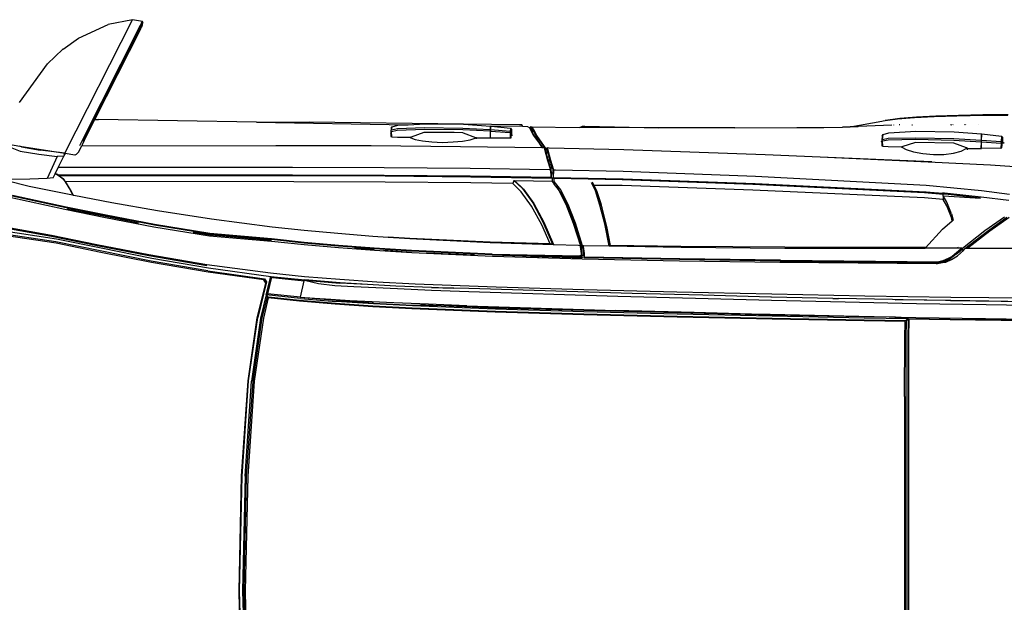
# Model space of a CAD drawing. Units: inches. Extents: x 22042254 to 25404563, y 17568978 to 17626777.
# Tile 15 of 45: x 22042341.458 to 22042342.604, y 17568978.204 to 17568978.882. Entities that reach past the tile are written whole.
import ezdxf

# ---------------------------------------------------------------- set-up
doc = ezdxf.new("R2010")
doc.units = ezdxf.units.IN
doc.header["$MEASUREMENT"] = 0
doc.layers.add('A-SITE-VEHI', color=8, linetype='Continuous', lineweight=18)
doc.layers.add('Edges', color=250, linetype='Continuous')

# ---------------------------------------------------------------- blocks, each defined once
blk = doc.blocks.new('Nissan Qashqai pl')
at = {"layer": 'Edges'}
for p, q in [((10.4706, 11.5566), (10.4706, 12.2875)), ((10.4726, 11.5567), (10.4726, 12.2875)), ((10.4764, 11.5569), (10.4764, 12.2872)), ((10.4776, 11.5567), (10.4776, 12.2874)), ((9.2241, 12.1376), (9.2195, 11.9221)), ((9.2249, 12.1376), (9.2203, 11.9221)), ((9.2259, 11.9221), (9.2305, 12.1375)), ((9.2335, 12.1374), (9.2289, 11.9221)), ((9.2308, 11.9221), (9.2355, 12.1374)), ((9.2195, 11.9221), (9.2241, 11.7066)), ((9.2203, 11.9221), (9.2249, 11.7065)), ((9.2305, 11.7067), (9.2259, 11.9221)), ((9.2289, 11.9221), (9.2335, 11.7067)), ((9.2355, 11.7068), (9.2308, 11.9221)), ((9.2241, 11.7066), (9.2362, 11.5274)), ((9.2249, 11.7065), (9.2371, 11.5273)), ((9.2305, 11.7067), (9.2426, 11.5277)), ((9.2335, 11.7067), (9.2457, 11.5277)), ((9.2476, 11.5278), (9.2355, 11.7068)), ((10.4706, 11.5566), (10.4711, 11.4469)), ((10.4731, 11.4469), (10.4726, 11.5567)), ((10.4769, 11.4474), (10.4764, 11.5569)), ((10.4781, 11.4469), (10.4776, 11.5567)), ((9.2362, 11.5274), (9.2535, 11.4087)), ((9.2371, 11.5273), (9.2543, 11.4085)), ((9.2598, 11.4093), (9.2426, 11.5277)), ((9.2457, 11.5277), (9.2629, 11.4092)), ((9.2649, 11.4094), (9.2476, 11.5278)), ((10.4711, 11.4469), (10.4715, 11.416)), ((10.4735, 11.414), (10.4731, 11.4469)), ((10.4773, 11.4146), (10.4769, 11.4474)), ((10.4785, 11.4111), (10.4781, 11.4469)), ((9.2535, 11.4087), (9.2694, 11.3436)), ((9.2707, 11.3414), (9.2543, 11.4085)), ((9.2704, 11.3659), (9.2598, 11.4093)), ((9.2629, 11.4092), (9.2726, 11.3695)), ((9.2741, 11.3716), (9.2649, 11.4094)), ((10.0431, 11.4075), (9.8673, 11.4031)), ((9.8673, 11.4012), (10.043, 11.4055)), ((10.2215, 11.406), (10.0429, 11.4021)), ((10.2216, 11.4037), (10.0429, 11.3998)), ((10.043, 11.4055), (10.2218, 11.4094)), ((10.2218, 11.4114), (10.0431, 11.4075)), ((10.3564, 11.406), (10.2175, 11.4028)), ((10.3945, 11.4094), (10.2215, 11.406)), ((10.3947, 11.4071), (10.2216, 11.4037)), ((10.3947, 11.4148), (10.2218, 11.4114)), ((10.2218, 11.4094), (10.3947, 11.4128)), ((10.4416, 11.4077), (10.3564, 11.406)), ((10.4773, 11.4107), (10.3945, 11.4094)), ((10.4715, 11.416), (10.3947, 11.4148)), ((10.3947, 11.4128), (10.4735, 11.414)), ((10.4416, 11.4078), (10.3947, 11.4071)), ((10.4519, 11.4079), (10.4416, 11.4077)), ((10.4519, 11.4079), (10.4416, 11.4078)), ((10.4416, 11.4077), (10.4416, 11.4078)), ((10.4524, 11.408), (10.4519, 11.4079)), ((10.4519, 11.4079), (10.4519, 11.4079)), ((10.4524, 11.4079), (10.4519, 11.4079)), ((10.4524, 11.4079), (10.4524, 11.408)), ((10.4533, 11.408), (10.4524, 11.408)), ((10.4533, 11.4079), (10.4524, 11.4079)), ((10.4638, 11.4081), (10.4533, 11.4079)), ((10.4638, 11.4081), (10.4533, 11.408)), ((10.4533, 11.4079), (10.4533, 11.408)), ((10.4914, 11.4087), (10.4638, 11.4081)), ((10.4773, 11.4107), (10.4735, 11.414)), ((10.4773, 11.4146), (10.4773, 11.4107)), ((10.4773, 11.4107), (10.5561, 11.4119)), ((10.4773, 11.4107), (10.4785, 11.4111)), ((10.5563, 11.4123), (10.4785, 11.4111)), ((10.6223, 11.4109), (10.4914, 11.4087)), ((10.6996, 11.4134), (10.5561, 11.4119)), ((10.5563, 11.4123), (10.6999, 11.4138)), ((10.7493, 11.4125), (10.6223, 11.4109)), ((9.4706, 11.388), (9.4, 11.3832)), ((9.4004, 11.3813), (9.4709, 11.3861)), ((9.5443, 11.3919), (9.4706, 11.388)), ((9.4709, 11.3861), (9.5446, 11.39)), ((9.5454, 11.3866), (9.472, 11.3828)), ((9.472, 11.3812), (9.5454, 11.3851)), ((9.701, 11.3983), (9.5443, 11.3919)), ((9.5446, 11.39), (9.7011, 11.3963)), ((9.7014, 11.3929), (9.5454, 11.3866)), ((9.5454, 11.3851), (9.5695, 11.3853)), ((9.5454, 11.3848), (9.5454, 11.3851)), ((9.5695, 11.3853), (9.5609, 11.3849)), ((9.7014, 11.3906), (9.5695, 11.3853)), ((9.5695, 11.3853), (9.5786, 11.3853)), ((9.6472, 11.3861), (9.5755, 11.3834)), ((9.5786, 11.3853), (9.6206, 11.3861)), ((9.6206, 11.3861), (9.6714, 11.3874)), ((9.6472, 11.3861), (9.9278, 11.3949)), ((9.6714, 11.3874), (9.8565, 11.3931)), ((9.8673, 11.4031), (9.701, 11.3983)), ((9.7011, 11.3963), (9.8673, 11.4012)), ((9.8673, 11.3977), (9.7014, 11.3929)), ((9.8673, 11.3954), (9.7014, 11.3906)), ((9.8565, 11.3931), (9.9794, 11.3967)), ((10.0429, 11.4021), (9.8673, 11.3977)), ((10.0429, 11.3998), (9.8673, 11.3954)), ((10.0747, 11.3991), (9.9278, 11.3949)), ((9.9794, 11.3967), (10.0965, 11.3998)), ((10.2043, 11.4025), (10.0747, 11.3991)), ((10.0965, 11.3998), (10.0998, 11.3999)), ((10.0998, 11.3999), (10.2043, 11.4025)), ((10.2175, 11.4028), (10.2043, 11.4025)), ((10.6237, 11.3839), (10.7502, 11.3855)), ((9.3346, 11.3724), (9.2704, 11.3659)), ((9.2704, 11.3659), (9.2726, 11.3695)), ((9.3346, 11.37), (9.2724, 11.3637)), ((9.2726, 11.3695), (9.2746, 11.3697)), ((9.3326, 11.3776), (9.2741, 11.3716)), ((9.2746, 11.3697), (9.333, 11.3757)), ((9.4, 11.3832), (9.3326, 11.3776)), ((9.333, 11.3757), (9.4004, 11.3813)), ((9.4017, 11.3765), (9.3344, 11.3708)), ((9.3611, 11.3727), (9.3344, 11.3708)), ((9.3344, 11.3708), (9.3346, 11.37)), ((9.3346, 11.3724), (9.4018, 11.378)), ((9.3346, 11.37), (9.3418, 11.3391)), ((9.3918, 11.3747), (9.3611, 11.3727)), ((9.4276, 11.3767), (9.3918, 11.3747)), ((9.472, 11.3812), (9.4017, 11.3765)), ((9.472, 11.3828), (9.4018, 11.378)), ((9.4694, 11.3788), (9.4276, 11.3767)), ((9.5105, 11.3805), (9.4694, 11.3788)), ((9.5755, 11.3834), (9.5105, 11.3805)), ((9.6514, 11.3592), (9.9312, 11.3681)), ((9.9312, 11.3681), (10.0776, 11.3722)), ((10.091, 11.3666), (9.9583, 11.363)), ((10.0776, 11.3722), (10.2201, 11.3759)), ((10.2191, 11.3699), (10.091, 11.3666)), ((10.2202, 11.3699), (10.2191, 11.3699)), ((10.2201, 11.3759), (10.3586, 11.3791)), ((10.2202, 11.3699), (10.2203, 11.3699)), ((10.3353, 11.3725), (10.2203, 11.3699)), ((10.3955, 11.368), (10.2211, 11.3646)), ((10.3353, 11.3725), (10.346, 11.3727)), ((10.4477, 11.3747), (10.346, 11.3727)), ((10.3586, 11.3791), (10.4931, 11.3817)), ((10.5572, 11.3704), (10.3955, 11.368)), ((10.4537, 11.3749), (10.4477, 11.3747)), ((10.4537, 11.3749), (10.4538, 11.3749)), ((10.4681, 11.3752), (10.4538, 11.3749)), ((10.4676, 11.3751), (10.4538, 11.3749)), ((10.5576, 11.3766), (10.4676, 11.3751)), ((10.5566, 11.3765), (10.4676, 11.3751)), ((10.4676, 11.3751), (10.4676, 11.3751)), ((10.5866, 11.3772), (10.4681, 11.3752)), ((10.4931, 11.3817), (10.6237, 11.3839)), ((10.5566, 11.3765), (10.7, 11.378)), ((10.7004, 11.372), (10.5572, 11.3704)), ((10.6649, 11.3783), (10.5576, 11.3766)), ((10.6649, 11.3783), (10.5866, 11.3772)), ((9.2704, 11.3659), (9.2724, 11.3637)), ((9.2704, 11.3659), (9.2789, 11.331)), ((9.2799, 11.3328), (9.2724, 11.3637)), ((9.3687, 11.3441), (9.3992, 11.3482)), ((9.3992, 11.3482), (9.4347, 11.3502)), ((9.4347, 11.3502), (9.4761, 11.3522)), ((9.514, 11.3492), (9.4605, 11.3465)), ((9.4761, 11.3522), (9.5168, 11.3539)), ((9.5811, 11.3522), (9.514, 11.3492)), ((9.5168, 11.3539), (9.5812, 11.3568)), ((9.7029, 11.3516), (9.5503, 11.3455)), ((9.5811, 11.3522), (9.6231, 11.3531)), ((9.594, 11.3527), (9.5811, 11.3522)), ((9.5812, 11.3568), (9.6514, 11.3592)), ((9.6231, 11.3531), (9.594, 11.3527)), ((9.651, 11.3536), (9.6231, 11.3531)), ((9.9583, 11.363), (9.651, 11.3536)), ((9.8673, 11.3563), (9.7029, 11.3516)), ((10.0423, 11.3607), (9.8673, 11.3563)), ((10.2211, 11.3646), (10.0423, 11.3607)), ((9.1605, 11.3208), (9.2669, 11.3354)), ((9.2656, 11.3376), (9.1612, 11.3233)), ((9.1617, 11.315), (9.2789, 11.331)), ((9.2694, 11.3436), (9.2656, 11.3376)), ((9.2669, 11.3354), (9.2656, 11.3376)), ((9.2669, 11.3354), (9.2707, 11.3414)), ((9.2694, 11.3436), (9.2707, 11.3414)), ((9.3422, 11.3316), (9.2783, 11.3251)), ((9.2789, 11.331), (9.3427, 11.3375)), ((9.2789, 11.331), (9.2799, 11.3327)), ((9.2799, 11.3328), (9.2819, 11.333)), ((9.2799, 11.3327), (9.2799, 11.3328)), ((9.2799, 11.3327), (9.2811, 11.3325)), ((9.2819, 11.333), (9.3418, 11.3391)), ((9.3418, 11.3391), (9.342, 11.3383)), ((9.342, 11.3383), (9.3687, 11.3441)), ((9.342, 11.3383), (9.4087, 11.3438)), ((9.4088, 11.3371), (9.3422, 11.3316)), ((9.4093, 11.3431), (9.3427, 11.3375)), ((9.4605, 11.3465), (9.4087, 11.3438)), ((9.4782, 11.3418), (9.4088, 11.3371)), ((9.4605, 11.3465), (9.4093, 11.3431)), ((9.5503, 11.3455), (9.4782, 11.3418)), ((9.1605, 11.3208), (9.0538, 11.3023)), ((9.1612, 11.3233), (9.0546, 11.3048)), ((9.0552, 11.2965), (9.1617, 11.315)), ((9.2783, 11.3251), (9.1584, 11.3091)), ((9.0538, 11.3023), (8.9583, 11.2833)), ((9.0546, 11.3048), (8.9591, 11.2859)), ((8.9598, 11.2775), (9.0552, 11.2965)), ((9.1584, 11.3091), (9.0495, 11.2906)), ((9.0497, 11.2918), (9.1586, 11.3104)), ((9.5443, 11.2863), (9.696, 11.2932)), ((9.6953, 11.2892), (9.863, 11.2944)), ((9.6953, 11.2892), (9.8598, 11.2925)), ((9.6954, 11.2907), (9.8641, 11.2959)), ((9.696, 11.2932), (9.8644, 11.2982)), ((9.7669, 11.2945), (9.7832, 11.2951)), ((9.8629, 11.2925), (9.8598, 11.2925)), ((9.8627, 11.2909), (9.8629, 11.2925)), ((9.8629, 11.2925), (9.863, 11.2944)), ((9.8641, 11.2959), (9.863, 11.2944)), ((9.8637, 11.291), (9.8638, 11.2934)), ((9.8638, 11.2934), (9.8641, 11.2959)), ((9.8644, 11.2982), (10.0472, 11.3018)), ((9.8678, 11.2935), (9.8677, 11.291)), ((9.8681, 11.2959), (9.8678, 11.2935)), ((10.0476, 11.2996), (9.8681, 11.2959)), ((9.8681, 11.2959), (9.869, 11.2946)), ((9.8689, 11.2927), (9.8686, 11.2879)), ((9.869, 11.2946), (9.8689, 11.2927)), ((10.0477, 11.2982), (9.869, 11.2946)), ((10.0472, 11.3018), (10.2357, 11.3043)), ((10.2367, 11.3022), (10.0476, 11.2996)), ((10.2369, 11.3008), (10.0477, 11.2982)), ((10.2357, 11.3043), (10.53, 11.3068)), ((10.2367, 11.3022), (10.5351, 11.305)), ((10.2369, 11.3008), (10.5348, 11.3036)), ((10.4153, 11.3058), (10.2954, 11.3046)), ((10.4153, 11.3058), (10.4174, 11.3058)), ((10.4174, 11.3058), (10.4181, 11.3058)), ((10.4181, 11.3058), (10.4182, 11.3058)), ((10.4182, 11.3058), (10.53, 11.3068)), ((10.53, 11.3068), (10.5301, 11.3068)), ((10.5301, 11.3068), (10.5323, 11.3065)), ((10.5323, 11.3065), (10.5419, 11.3051)), ((10.5422, 11.3021), (10.5348, 11.3036)), ((10.5424, 11.3035), (10.5351, 11.305)), ((10.5366, 11.3048), (10.536, 11.305)), ((10.5379, 11.3052), (10.5381, 11.305)), ((10.5419, 11.3051), (10.5463, 11.3031)), ((10.5419, 11.3051), (10.5479, 11.3042)), ((10.5522, 11.2977), (10.5422, 11.3021)), ((10.5472, 11.3014), (10.5424, 11.3035)), ((10.5463, 11.3031), (10.5551, 11.2984)), ((10.5546, 11.2982), (10.5472, 11.3014)), ((10.5479, 11.3042), (10.5589, 11.2991)), ((10.5598, 11.2935), (10.5522, 11.2977)), ((10.5583, 11.296), (10.5546, 11.2982)), ((10.5551, 11.2984), (10.5583, 11.296)), ((10.5612, 11.2944), (10.5583, 11.296)), ((10.5589, 11.2991), (10.57, 11.2925)), ((10.5764, 11.28), (10.5598, 11.2935)), ((10.5683, 11.2885), (10.5612, 11.2944)), ((10.57, 11.2925), (10.5811, 11.2822)), ((8.9583, 11.2833), (8.8745, 11.266)), ((8.9591, 11.2859), (8.8754, 11.2687)), ((8.8761, 11.2602), (8.9598, 11.2775)), ((9.0495, 11.2906), (8.9521, 11.2715)), ((8.9522, 11.2728), (9.0497, 11.2918)), ((9.3418, 11.2713), (9.4064, 11.277)), ((9.4063, 11.2743), (9.3419, 11.2685)), ((9.4735, 11.2779), (9.4062, 11.2729)), ((9.4736, 11.2793), (9.4063, 11.2743)), ((9.4064, 11.277), (9.4739, 11.282)), ((9.4727, 11.2808), (9.4362, 11.278)), ((9.4727, 11.2808), (9.4732, 11.2808)), ((9.5437, 11.2822), (9.4735, 11.2779)), ((9.5438, 11.2836), (9.4736, 11.2793)), ((9.4739, 11.282), (9.5443, 11.2863)), ((9.491, 11.2819), (9.5434, 11.2852)), ((9.6953, 11.2892), (9.5437, 11.2822)), ((9.6954, 11.2907), (9.5438, 11.2836)), ((9.5717, 11.2865), (9.6618, 11.2907)), ((9.8652, 11.2788), (9.8516, 11.2363)), ((9.8603, 11.2727), (9.8605, 11.2746)), ((9.8605, 11.2746), (9.8626, 11.2878)), ((9.8612, 11.2735), (9.8615, 11.2754)), ((9.8615, 11.2754), (9.8635, 11.2886)), ((9.8626, 11.2878), (9.8627, 11.2909)), ((9.8627, 11.2909), (9.8637, 11.291)), ((9.8635, 11.2886), (9.8637, 11.291)), ((9.8637, 11.291), (9.8643, 11.291)), ((9.8643, 11.291), (9.8677, 11.291)), ((9.8652, 11.2738), (9.8652, 11.2788)), ((9.8655, 11.2754), (9.8652, 11.2738)), ((9.8652, 11.2735), (9.8665, 11.2747)), ((9.8675, 11.2887), (9.8655, 11.2754)), ((9.8665, 11.2747), (9.8664, 11.2728)), ((9.8686, 11.2879), (9.8665, 11.2747)), ((9.8677, 11.291), (9.8675, 11.2887)), ((9.9149, 11.2736), (10.0505, 11.276)), ((10.0501, 11.2747), (9.9177, 11.2728)), ((10.2453, 11.2762), (10.0501, 11.2747)), ((10.0505, 11.276), (10.2453, 11.2777)), ((10.2453, 11.2777), (10.4289, 11.2783)), ((10.4292, 11.2767), (10.2453, 11.2762)), ((10.4289, 11.2783), (10.5092, 11.2783)), ((10.5099, 11.2768), (10.4292, 11.2767)), ((10.5099, 11.2768), (10.5092, 11.2783)), ((10.5092, 11.2783), (10.5094, 11.2783)), ((10.5094, 11.2783), (10.51, 11.2776)), ((10.5783, 11.2783), (10.5094, 11.2783)), ((10.51, 11.2776), (10.5099, 11.2768)), ((10.51, 11.2776), (10.5419, 11.2423)), ((10.5683, 11.2885), (10.573, 11.285)), ((10.575, 11.2829), (10.5683, 11.2885)), ((10.5705, 11.2771), (10.5709, 11.2767)), ((10.5709, 11.2767), (10.5719, 11.2759)), ((10.573, 11.285), (10.5769, 11.2818)), ((10.5776, 11.2808), (10.575, 11.2829)), ((10.5783, 11.2783), (10.5764, 11.28)), ((10.5796, 11.2787), (10.5776, 11.2808)), ((10.5776, 11.2808), (10.5783, 11.2783)), ((10.5796, 11.2787), (10.5783, 11.2783)), ((10.5796, 11.2824), (10.5796, 11.2787)), ((10.6215, 11.2456), (10.5796, 11.2787)), ((10.5811, 11.2822), (10.5821, 11.2808)), ((10.5811, 11.2822), (10.5834, 11.28)), ((10.5821, 11.2808), (10.5834, 11.2793)), ((10.5825, 11.2806), (10.5834, 11.2793)), ((10.5834, 11.28), (10.5851, 11.2783)), ((10.5834, 11.2793), (10.5835, 11.2793)), ((10.5835, 11.2793), (10.584, 11.2787)), ((10.584, 11.2789), (10.584, 11.2793)), ((10.584, 11.2787), (10.584, 11.2789)), ((10.584, 11.2787), (10.6261, 11.2458)), ((10.584, 11.2787), (10.5851, 11.2783)), ((10.5843, 11.2787), (10.584, 11.2787)), ((10.5847, 11.2787), (10.5843, 11.2787)), ((10.5851, 11.2783), (10.5892, 11.2783)), ((10.6306, 11.2459), (10.5892, 11.2783)), ((10.5892, 11.2783), (10.6988, 11.2779)), ((8.7287, 11.2307), (8.8666, 11.2554)), ((8.8745, 11.266), (8.7481, 11.2473)), ((8.8754, 11.2687), (8.7491, 11.2501)), ((8.7496, 11.2416), (8.8761, 11.2602)), ((8.8666, 11.2554), (8.9522, 11.2728)), ((8.9521, 11.2715), (8.8666, 11.2541)), ((9.1639, 11.2546), (9.2801, 11.2648)), ((9.2803, 11.2606), (9.1644, 11.2503)), ((9.2804, 11.262), (9.1645, 11.2518)), ((9.2804, 11.2635), (9.1668, 11.2533)), ((9.2801, 11.2648), (9.3418, 11.2713)), ((9.3418, 11.2671), (9.2803, 11.2606)), ((9.3419, 11.2685), (9.2804, 11.262)), ((9.4062, 11.2729), (9.3418, 11.2671)), ((9.4048, 11.2501), (9.471, 11.2554)), ((9.471, 11.2554), (9.4997, 11.2573)), ((9.4997, 11.2573), (9.5403, 11.26)), ((9.5404, 11.2598), (9.4997, 11.2573)), ((9.5403, 11.26), (9.6913, 11.2674)), ((9.6912, 11.2667), (9.5404, 11.2598)), ((9.8039, 11.27), (9.6912, 11.2667)), ((9.6913, 11.2674), (9.8099, 11.2711)), ((9.8039, 11.27), (9.7884, 11.2343)), ((9.7905, 11.2283), (9.8087, 11.2702)), ((9.7925, 11.2294), (9.8107, 11.2711)), ((9.8087, 11.2702), (9.8039, 11.27)), ((9.8099, 11.2711), (9.8087, 11.2702)), ((9.8099, 11.2711), (9.8107, 11.2711)), ((9.8107, 11.2711), (9.8573, 11.2726)), ((9.8475, 11.2312), (9.8611, 11.2734)), ((9.8652, 11.2738), (9.8516, 11.2313)), ((9.8573, 11.2726), (9.8603, 11.2727)), ((9.8611, 11.2734), (9.8603, 11.2727)), ((9.8612, 11.2735), (9.8611, 11.2734)), ((9.8652, 11.2738), (9.8652, 11.2738)), ((9.8652, 11.2738), (9.8652, 11.2735)), ((9.8652, 11.2735), (9.8664, 11.2728)), ((9.8664, 11.2728), (9.9149, 11.2736)), ((9.9149, 11.2736), (9.9066, 11.2322)), ((9.9169, 11.2728), (9.9086, 11.2313)), ((9.9177, 11.2728), (9.9106, 11.2373)), ((9.9177, 11.2728), (9.9169, 11.2728)), ((8.8666, 11.2541), (8.7292, 11.2295)), ((8.9679, 11.2201), (9.0591, 11.2377)), ((9.0591, 11.2377), (9.1639, 11.2546)), ((9.1644, 11.2503), (9.06, 11.2335)), ((9.1645, 11.2518), (9.0601, 11.235)), ((9.133, 11.2481), (9.1647, 11.2532)), ((9.1647, 11.2532), (9.1668, 11.2533)), ((9.1676, 11.2229), (9.2814, 11.2377)), ((9.2814, 11.2377), (9.3416, 11.2442)), ((9.3416, 11.2442), (9.4048, 11.2501)), ((9.9106, 11.2373), (9.9018, 11.2021)), ((10.5419, 11.2423), (10.56, 11.2265)), ((10.6583, 11.2197), (10.6215, 11.2456)), ((10.6261, 11.2458), (10.6627, 11.22)), ((10.6671, 11.2203), (10.6306, 11.2459)), ((8.8918, 11.205), (8.9679, 11.2201)), ((9.0601, 11.235), (8.8941, 11.2023)), ((8.9318, 11.211), (8.9704, 11.2185)), ((9.06, 11.2335), (8.9696, 11.2157)), ((8.9704, 11.2185), (8.9708, 11.2185)), ((8.9708, 11.2185), (9.03, 11.2304)), ((9.0656, 11.207), (9.1676, 11.2229)), ((9.7884, 11.2343), (9.7692, 11.1989)), ((9.7713, 11.1929), (9.7905, 11.2283)), ((9.7733, 11.194), (9.7925, 11.2294)), ((9.8338, 11.1956), (9.8475, 11.2312)), ((9.8516, 11.2363), (9.8378, 11.2007)), ((9.8516, 11.2313), (9.8378, 11.1957)), ((9.9066, 11.2322), (9.8978, 11.197)), ((9.9086, 11.2313), (9.8998, 11.196)), ((10.5584, 11.2206), (10.5502, 11.1986)), ((10.56, 11.2265), (10.5584, 11.2206)), ((10.5584, 11.2136), (10.5617, 11.2251)), ((10.56, 11.2265), (10.5617, 11.2251)), ((8.7881, 11.1821), (8.8918, 11.205)), ((8.8941, 11.2023), (8.7925, 11.1802)), ((8.8942, 11.2009), (8.7931, 11.1789)), ((8.9696, 11.2157), (8.8942, 11.2009)), ((8.8961, 11.204), (8.9318, 11.211)), ((8.9797, 11.1924), (9.0656, 11.207)), ((9.8378, 11.2007), (9.8241, 11.1736)), ((9.9018, 11.2021), (9.8931, 11.1752)), ((10.5584, 11.2136), (10.5502, 11.1916)), ((8.9087, 11.1783), (8.9797, 11.1924)), ((9.7692, 11.1989), (9.7499, 11.1721)), ((9.7519, 11.1661), (9.7713, 11.1929)), ((9.754, 11.1672), (9.7733, 11.194)), ((9.8201, 11.1685), (9.8338, 11.1956)), ((9.8378, 11.1957), (9.8241, 11.1686)), ((9.8978, 11.197), (9.8891, 11.1701)), ((9.8911, 11.1693), (9.8998, 11.196)), ((10.5079, 11.1835), (10.1849, 11.1687)), ((10.543, 11.1865), (10.5079, 11.1835)), ((10.5502, 11.1986), (10.543, 11.1865)), ((10.5502, 11.1916), (10.543, 11.1795)), ((10.543, 11.1795), (10.543, 11.1865)), ((10.5439, 11.1796), (10.613, 11.1841)), ((10.5458, 11.1742), (10.6144, 11.1813)), ((10.613, 11.1841), (10.547, 11.1767)), ((10.6144, 11.1813), (10.6664, 11.1875)), ((8.8245, 11.1613), (8.9063, 11.1779)), ((8.8893, 11.1486), (8.9021, 11.1697)), ((8.9041, 11.1717), (8.8927, 11.1528)), ((8.9021, 11.1697), (8.9063, 11.1779)), ((8.9075, 11.1781), (8.9041, 11.1717)), ((8.9063, 11.1779), (8.9075, 11.1781)), ((8.9075, 11.1781), (8.9087, 11.1783)), ((9.7499, 11.1721), (9.7337, 11.1566)), ((9.7357, 11.1507), (9.7519, 11.1661)), ((9.7378, 11.1517), (9.754, 11.1672)), ((9.8241, 11.1686), (9.8119, 11.1529)), ((9.8241, 11.1736), (9.8147, 11.1616)), ((9.8147, 11.1616), (9.8201, 11.1685)), ((9.8891, 11.1701), (9.8818, 11.1551)), ((9.8911, 11.1691), (9.8867, 11.16)), ((9.8931, 11.1751), (9.8911, 11.1693)), ((9.8911, 11.1693), (9.8911, 11.1691)), ((9.8931, 11.1751), (9.8931, 11.1752)), ((10.1849, 11.1687), (9.9393, 11.1602)), ((10.5079, 11.1739), (10.1849, 11.1585)), ((10.1894, 11.1563), (10.5109, 11.1721)), ((10.543, 11.1771), (10.5079, 11.1739)), ((10.5109, 11.1721), (10.5417, 11.1748)), ((10.6152, 11.1702), (10.5113, 11.1603)), ((10.543, 11.1771), (10.5417, 11.1748)), ((10.5417, 11.1748), (10.5427, 11.1739)), ((10.5436, 11.1754), (10.5427, 11.1739)), ((10.5427, 11.1739), (10.5458, 11.1742)), ((10.5439, 11.1796), (10.543, 11.1795)), ((10.543, 11.1795), (10.543, 11.1771)), ((10.544, 11.1763), (10.543, 11.1771)), ((10.544, 11.1763), (10.5436, 11.1754)), ((10.547, 11.1767), (10.544, 11.1763)), ((10.6678, 11.177), (10.6152, 11.1702)), ((8.7828, 11.1508), (8.8245, 11.1613)), ((8.8259, 11.1483), (8.7916, 11.1488)), ((8.8585, 11.1473), (8.8259, 11.1483)), ((8.87, 11.1455), (8.8585, 11.1473)), ((8.8771, 11.1054), (8.8585, 11.1473)), ((8.87, 11.1455), (8.8734, 11.1385)), ((8.8893, 11.1486), (8.8751, 11.1387)), ((8.881, 11.1418), (8.8893, 11.1486)), ((8.8913, 11.1506), (8.8893, 11.1486)), ((8.8927, 11.1528), (8.8913, 11.1506)), ((9.3225, 11.1531), (8.8927, 11.1528)), ((9.4936, 11.1538), (9.3225, 11.1531)), ((9.6552, 11.1554), (9.4936, 11.1538)), ((9.6552, 11.1445), (9.4936, 11.1428)), ((9.654, 11.1423), (9.8061, 11.1447)), ((9.7337, 11.1566), (9.6552, 11.1554)), ((9.8078, 11.1471), (9.6552, 11.1445)), ((9.7357, 11.1507), (9.7337, 11.1566)), ((9.7357, 11.1507), (9.7378, 11.1517)), ((9.8078, 11.1528), (9.7378, 11.1517)), ((9.8061, 11.1447), (9.8051, 11.1309)), ((9.8058, 11.1369), (9.8061, 11.1447)), ((9.8061, 11.1447), (9.8078, 11.1471)), ((9.8078, 11.1528), (9.8119, 11.1579)), ((9.8078, 11.1471), (9.8078, 11.1528)), ((9.8101, 11.1449), (9.8098, 11.1369)), ((9.8101, 11.1449), (9.9411, 11.1475)), ((9.8119, 11.1472), (9.8101, 11.1449)), ((9.8101, 11.1449), (9.8112, 11.1311)), ((9.8147, 11.1616), (9.8119, 11.1579)), ((9.8119, 11.1579), (9.8119, 11.1529)), ((9.8119, 11.1529), (9.8119, 11.1472)), ((9.9393, 11.1497), (9.8119, 11.1472)), ((9.8147, 11.1616), (9.8147, 11.1616)), ((9.8867, 11.16), (9.8838, 11.1541)), ((9.9393, 11.1602), (9.8867, 11.16)), ((10.1849, 11.1585), (9.9393, 11.1497)), ((9.9411, 11.1475), (10.1894, 11.1563)), ((10.5113, 11.1603), (10.19, 11.1433)), ((8.8734, 11.1385), (8.8793, 11.1261)), ((8.8734, 11.1385), (8.8768, 11.1385)), ((8.8751, 11.1387), (8.8768, 11.1385)), ((8.8768, 11.1385), (8.879, 11.1402)), ((8.879, 11.1402), (8.881, 11.1418)), ((8.879, 11.1402), (9.3198, 11.1403)), ((9.3194, 11.1262), (8.8793, 11.1261)), ((8.8793, 11.1261), (8.8815, 11.1214)), ((9.3225, 11.1421), (8.881, 11.1418)), ((9.4919, 11.1269), (9.3194, 11.1262)), ((9.3198, 11.1403), (9.4922, 11.1409)), ((9.4936, 11.1428), (9.3225, 11.1421)), ((9.6538, 11.1284), (9.4919, 11.1269)), ((9.4922, 11.1409), (9.654, 11.1423)), ((9.802, 11.1309), (9.6538, 11.1284)), ((9.7992, 11.1133), (9.8044, 11.129)), ((9.8051, 11.1309), (9.802, 11.1309)), ((9.8041, 11.1256), (9.8045, 11.1268)), ((9.8044, 11.129), (9.8051, 11.1309)), ((9.8045, 11.1268), (9.8046, 11.1271)), ((9.8045, 11.1268), (9.8085, 11.1268)), ((9.8046, 11.1271), (9.8055, 11.1298)), ((9.8086, 11.1271), (9.8046, 11.1271)), ((9.8106, 11.1292), (9.8054, 11.1135)), ((9.8055, 11.1298), (9.8058, 11.1369)), ((9.8098, 11.1369), (9.8058, 11.1369)), ((9.8085, 11.1268), (9.8081, 11.1256)), ((9.8086, 11.1271), (9.8085, 11.1268)), ((9.8096, 11.13), (9.8086, 11.1271)), ((9.8098, 11.1369), (9.8096, 11.13)), ((9.8112, 11.1311), (9.8106, 11.1292)), ((9.8143, 11.1312), (9.8112, 11.1311)), ((9.9414, 11.1341), (9.8143, 11.1312)), ((10.19, 11.1433), (9.9414, 11.1341)), ((10.6318, 11.1213), (10.6955, 11.1257)), ((8.8815, 11.1214), (8.892, 11.0998)), ((8.8815, 11.1214), (8.8895, 11.1048)), ((9.7937, 11.0918), (9.7992, 11.1133)), ((9.7978, 11.1044), (9.7987, 11.108)), ((9.7987, 11.108), (9.8002, 11.1141)), ((9.7992, 11.1065), (9.7987, 11.108)), ((9.8027, 11.1078), (9.7992, 11.1065)), ((9.8054, 11.1135), (9.7999, 11.0919)), ((9.8002, 11.1141), (9.8008, 11.1157)), ((9.8027, 11.1078), (9.8003, 11.0983)), ((9.8008, 11.1157), (9.8014, 11.1176)), ((9.8014, 11.1139), (9.8008, 11.1157)), ((9.803, 11.1212), (9.8014, 11.1176)), ((9.8014, 11.1176), (9.8026, 11.1212)), ((9.8043, 11.1139), (9.8014, 11.1139)), ((9.8031, 11.1093), (9.8014, 11.1139)), ((9.8026, 11.1212), (9.8041, 11.1256)), ((9.803, 11.1212), (9.8026, 11.1212)), ((9.8031, 11.1093), (9.8027, 11.1078)), ((9.8067, 11.1213), (9.803, 11.1212)), ((9.8043, 11.1139), (9.8031, 11.1093)), ((9.8041, 11.1256), (9.8081, 11.1256)), ((9.8044, 11.1142), (9.8043, 11.1139)), ((9.8067, 11.1213), (9.8044, 11.1142)), ((9.8081, 11.1256), (9.8067, 11.1213)), ((10.312, 11.1064), (10.5147, 11.1156)), ((10.312, 11.1064), (10.5214, 11.1149)), ((10.5147, 11.1156), (10.6318, 11.1213)), ((8.7917, 11.0895), (8.8075, 11.0955)), ((8.807, 11.0862), (8.8918, 11.0997)), ((8.8075, 11.0955), (8.8429, 11.1016)), ((8.8102, 11.0874), (8.8455, 11.0936)), ((8.8429, 11.1016), (8.8771, 11.1054)), ((8.8918, 11.0997), (8.8455, 11.0936)), ((8.8895, 11.1048), (8.8771, 11.1054)), ((8.8908, 11.1021), (8.8895, 11.1048)), ((8.8906, 11.1024), (8.8895, 11.1048)), ((8.8906, 11.1024), (8.8911, 11.1013)), ((8.892, 11.0998), (8.8908, 11.1021)), ((8.8911, 11.1013), (8.8919, 11.0997)), ((8.8911, 11.1013), (8.8919, 11.0998)), ((8.8919, 11.0997), (8.8911, 11.1013)), ((8.8919, 11.0997), (8.8918, 11.0997)), ((8.8918, 11.0997), (9.0186, 10.8486)), ((8.892, 11.0998), (8.8919, 11.0998)), ((8.8919, 11.0998), (8.8919, 11.0997)), ((8.8919, 11.0997), (8.8919, 11.0997)), ((8.9106, 11.1029), (8.892, 11.0998)), ((8.892, 11.0998), (8.892, 11.0998)), ((8.9131, 11.102), (8.9106, 11.1029)), ((8.9171, 11.0978), (8.9131, 11.102)), ((8.9171, 11.0978), (8.917, 11.0974)), ((8.9171, 11.0978), (8.9233, 11.0855)), ((9.6358, 11.0866), (9.7887, 11.0889)), ((9.7832, 11.0805), (9.7887, 11.0889)), ((9.7842, 11.0814), (9.7891, 11.0889)), ((9.7933, 11.0892), (9.7883, 11.0815)), ((9.7887, 11.0889), (9.7891, 11.0889)), ((9.7891, 11.0889), (9.79, 11.0889)), ((9.7965, 11.0915), (9.7894, 11.0806)), ((9.79, 11.0889), (9.7931, 11.089)), ((9.7931, 11.089), (9.7934, 11.0906)), ((9.7931, 11.089), (9.7933, 11.0892)), ((9.7933, 11.0892), (9.7941, 11.0901)), ((9.7934, 11.0906), (9.7937, 11.0918)), ((9.7934, 11.0906), (9.7938, 11.0904)), ((9.7941, 11.0901), (9.7943, 11.0907)), ((9.7964, 11.0988), (9.7943, 11.0907)), ((9.7955, 11.0925), (9.7943, 11.0907)), ((9.7963, 11.0918), (9.7955, 11.0925)), ((9.7992, 11.0966), (9.7963, 11.0918)), ((9.7963, 11.0918), (9.7963, 11.0918)), ((9.7964, 11.0917), (9.7963, 11.0918)), ((9.7964, 11.0988), (9.7973, 11.1023)), ((9.7964, 11.0988), (9.7992, 11.0966)), ((9.7964, 11.0917), (9.7996, 11.0966)), ((9.7964, 11.0917), (9.7964, 11.0917)), ((9.7967, 11.0915), (9.7964, 11.0917)), ((9.7965, 11.0915), (9.7967, 11.0915)), ((9.7983, 11.0901), (9.7965, 11.0915)), ((9.7967, 11.0915), (9.7986, 11.0916)), ((9.7977, 11.0907), (9.7967, 11.0915)), ((9.7973, 11.1023), (9.7977, 11.1042)), ((9.7977, 11.1033), (9.7973, 11.1023)), ((9.7973, 11.1023), (9.7977, 11.1011)), ((9.7987, 11.1053), (9.7977, 11.1033)), ((9.7977, 11.1042), (9.7978, 11.1044)), ((9.7977, 11.1042), (9.7977, 11.1033)), ((9.7977, 11.1011), (9.7977, 11.0998)), ((9.7977, 11.1011), (9.7985, 11.099)), ((9.7977, 11.0998), (9.7985, 11.099)), ((9.7982, 11.0902), (9.7977, 11.0907)), ((9.7987, 11.1053), (9.7978, 11.1044)), ((9.7986, 11.0916), (9.7982, 11.0902)), ((9.7983, 11.0901), (9.7982, 11.0902)), ((9.7986, 11.0898), (9.7983, 11.0901)), ((9.7985, 11.099), (9.7989, 11.098)), ((9.7988, 11.0925), (9.7986, 11.0916)), ((9.7986, 11.0898), (9.7993, 11.0891)), ((9.7992, 11.1065), (9.7987, 11.1053)), ((9.7998, 11.0964), (9.7988, 11.0925)), ((9.7989, 11.098), (9.7998, 11.0976)), ((9.7998, 11.0976), (9.7992, 11.0966)), ((9.7999, 11.0919), (9.7993, 11.0891)), ((9.7993, 11.0891), (9.8024, 11.0892)), ((9.8002, 11.098), (9.7996, 11.0966)), ((9.8001, 11.0974), (9.7996, 11.0966)), ((9.7996, 11.0966), (9.7998, 11.0964)), ((9.8003, 11.0983), (9.7998, 11.0976)), ((9.8001, 11.0974), (9.7998, 11.0964)), ((9.8002, 11.098), (9.8001, 11.0974)), ((9.8003, 11.0983), (9.8002, 11.098)), ((9.8024, 11.0892), (9.9426, 11.0923)), ((9.9426, 11.0923), (10.2081, 11.1017)), ((10.2081, 11.1017), (10.312, 11.1064)), ((10.4653, 11.0881), (10.4652, 11.0897)), ((10.4653, 11.0881), (10.4732, 11.0925)), ((10.4732, 11.0925), (10.4871, 11.0967)), ((10.4871, 11.0967), (10.5048, 11.1002)), ((10.5048, 11.1002), (10.5246, 11.1019)), ((10.5246, 11.1019), (10.5445, 11.1017)), ((10.5445, 11.1017), (10.5625, 11.0996)), ((10.5625, 11.0996), (10.5769, 11.0957)), ((10.5867, 11.0897), (10.563, 11.0809)), ((10.5769, 11.0957), (10.5863, 11.0904)), ((10.5863, 11.0904), (10.5867, 11.0897)), ((10.5885, 11.0904), (10.5867, 11.0897)), ((10.5885, 11.0931), (10.5885, 11.0904)), ((10.5885, 11.0904), (10.6141, 11.0905)), ((10.6141, 11.0905), (10.615, 11.0905)), ((10.6142, 11.0782), (10.6141, 11.0905)), ((10.6517, 11.0902), (10.615, 11.0905)), ((10.615, 11.0905), (10.6151, 11.0782)), ((10.6518, 11.0808), (10.6517, 11.0902)), ((10.6517, 11.0902), (10.6535, 11.0895)), ((10.6535, 11.0895), (10.6543, 11.0786)), ((10.6535, 11.0895), (10.6536, 11.0803)), ((8.7858, 11.0828), (8.807, 11.0862)), ((8.8102, 11.0874), (8.807, 11.0862)), ((8.9232, 11.0779), (8.9194, 11.0854)), ((9.0333, 10.8597), (8.9232, 11.0779)), ((8.9233, 11.0855), (9.2886, 11.0848)), ((8.925, 11.0821), (8.9233, 11.0855)), ((8.928, 11.0762), (8.925, 11.0821)), ((9.0386, 10.8534), (8.9254, 11.0778)), ((8.928, 11.0762), (8.9483, 11.0359)), ((9.2886, 11.0848), (9.4673, 11.0852)), ((9.4673, 11.0852), (9.6358, 11.0866)), ((9.5422, 11.0706), (9.5422, 11.0716)), ((9.5422, 11.0706), (9.5424, 11.0707)), ((9.5423, 11.0696), (9.5422, 11.0706)), ((9.5424, 11.0707), (9.5503, 11.0736)), ((9.5426, 11.0695), (9.5424, 11.0707)), ((9.5503, 11.0736), (9.5641, 11.076)), ((9.5641, 11.076), (9.5818, 11.0782)), ((9.5818, 11.0782), (9.6016, 11.0791)), ((9.6016, 11.0791), (9.6215, 11.0782)), ((9.6215, 11.0782), (9.6395, 11.0766)), ((9.6395, 11.0766), (9.654, 11.0744)), ((9.6645, 11.0705), (9.6413, 11.0616)), ((9.654, 11.0744), (9.6633, 11.0715)), ((9.6633, 11.0715), (9.6645, 11.0705)), ((9.6655, 11.0708), (9.6645, 11.0705)), ((9.6655, 11.0728), (9.6655, 11.0708)), ((9.6655, 11.0708), (9.6911, 11.0709)), ((9.6911, 11.0709), (9.692, 11.0709)), ((9.6911, 11.0645), (9.6911, 11.0709)), ((9.692, 11.0709), (9.692, 11.0645)), ((9.692, 11.0709), (9.7287, 11.0708)), ((9.7287, 11.0708), (9.7305, 11.0704)), ((9.7288, 11.0609), (9.7287, 11.0708)), ((9.7305, 11.0704), (9.7313, 11.0644)), ((9.7305, 11.0704), (9.7306, 11.0607)), ((9.7728, 11.066), (9.7832, 11.0805)), ((9.7738, 11.067), (9.7842, 11.0814)), ((9.7883, 11.0815), (9.7778, 11.0671)), ((9.7894, 11.0806), (9.7788, 11.0661)), ((10.4263, 11.0777), (10.4274, 11.0767)), ((10.4274, 11.0767), (10.4275, 11.0856)), ((10.4274, 11.0762), (10.4274, 11.0767)), ((10.4282, 11.0666), (10.4274, 11.0762)), ((10.4275, 11.0856), (10.4293, 11.0863)), ((10.4293, 11.0863), (10.4291, 11.0765)), ((10.4291, 11.0765), (10.4398, 11.0741)), ((10.4398, 11.0718), (10.4291, 11.0741)), ((10.4291, 11.0741), (10.4299, 11.0644)), ((10.4293, 11.0863), (10.4398, 11.0868)), ((10.4398, 11.0868), (10.4653, 11.0878)), ((10.4398, 11.0741), (10.4909, 11.0734)), ((10.4909, 11.0711), (10.4398, 11.0718)), ((10.4653, 11.0877), (10.4653, 11.0881)), ((10.4653, 11.0878), (10.4653, 11.0881)), ((10.4653, 11.0881), (10.4653, 11.0881)), ((10.4653, 11.0877), (10.4653, 11.0878)), ((10.4908, 11.0793), (10.4653, 11.0877)), ((10.563, 11.0809), (10.4908, 11.0793)), ((10.4909, 11.0734), (10.563, 11.075)), ((10.5631, 11.0727), (10.4909, 11.0711)), ((10.563, 11.075), (10.6142, 11.0779)), ((10.6142, 11.0756), (10.5631, 11.0727)), ((10.6142, 11.0779), (10.6142, 11.0782)), ((10.6142, 11.0765), (10.6142, 11.0779)), ((10.615, 11.0765), (10.6142, 11.0765)), ((10.6142, 11.0756), (10.6142, 11.0765)), ((10.615, 11.0639), (10.6142, 11.0756)), ((10.6151, 11.0765), (10.615, 11.0765)), ((10.615, 11.0765), (10.6151, 11.0639)), ((10.6151, 11.078), (10.6518, 11.0808)), ((10.6518, 11.0784), (10.6151, 11.0756)), ((10.6151, 11.0782), (10.6151, 11.078)), ((10.6151, 11.078), (10.6151, 11.0765)), ((10.6151, 11.0765), (10.6151, 11.0756)), ((10.6151, 11.0756), (10.616, 11.0629)), ((10.6518, 11.0784), (10.6518, 11.0808)), ((10.6518, 11.0808), (10.6536, 11.0803)), ((10.6536, 11.0803), (10.6518, 11.0784)), ((10.6526, 11.0674), (10.6518, 11.0784)), ((10.6536, 11.0803), (10.6537, 11.0783)), ((10.6543, 11.0786), (10.6537, 11.0783)), ((10.6537, 11.0783), (10.6543, 11.0693)), ((10.6578, 11.0814), (10.6543, 11.0786)), ((10.6543, 11.0693), (10.6543, 11.0786)), ((9.5037, 11.0635), (9.5045, 11.0628)), ((9.5044, 11.0586), (9.5045, 11.0628)), ((9.5052, 11.0524), (9.5044, 11.0586)), ((9.5045, 11.0683), (9.5063, 11.0687)), ((9.5045, 11.0628), (9.5045, 11.0683)), ((9.5052, 11.0524), (9.5069, 11.0501)), ((9.5063, 11.0687), (9.5061, 11.0586)), ((9.5061, 11.0586), (9.5167, 11.0559)), ((9.5168, 11.0537), (9.5061, 11.0564)), ((9.5061, 11.0564), (9.5069, 11.0501)), ((9.5063, 11.0687), (9.5168, 11.0691)), ((9.5167, 11.0559), (9.5679, 11.0543)), ((9.5168, 11.0691), (9.5423, 11.0696)), ((9.5679, 11.0521), (9.5168, 11.0537)), ((9.5426, 11.0695), (9.5423, 11.0696)), ((9.5667, 11.0609), (9.5426, 11.0695)), ((9.5678, 11.0604), (9.5667, 11.0609)), ((9.5846, 11.0606), (9.5678, 11.0604)), ((9.5679, 11.0543), (9.64, 11.0549)), ((9.6401, 11.0528), (9.5679, 11.0521)), ((9.6236, 11.0609), (9.5846, 11.0606)), ((9.64, 11.0611), (9.6236, 11.0609)), ((9.6413, 11.0616), (9.64, 11.0611)), ((9.64, 11.0549), (9.6912, 11.0577)), ((9.6913, 11.0556), (9.6401, 11.0528)), ((9.6912, 11.0631), (9.6911, 11.0645)), ((9.692, 11.0631), (9.6912, 11.0631)), ((9.6912, 11.0577), (9.6912, 11.0631)), ((9.6913, 11.0556), (9.6912, 11.0577)), ((9.692, 11.0499), (9.6913, 11.0556)), ((9.692, 11.0645), (9.692, 11.0631)), ((9.692, 11.0631), (9.6921, 11.0578)), ((9.6921, 11.0578), (9.7288, 11.0609)), ((9.6922, 11.0556), (9.6921, 11.0578)), ((9.7288, 11.0588), (9.6922, 11.0556)), ((9.6922, 11.0556), (9.693, 11.0486)), ((9.6922, 11.0556), (9.6922, 11.0499)), ((9.693, 11.0486), (9.7296, 11.0527)), ((9.7288, 11.0588), (9.7288, 11.0609)), ((9.7288, 11.0609), (9.7306, 11.0607)), ((9.7306, 11.0607), (9.7288, 11.0588)), ((9.7296, 11.0527), (9.7288, 11.0588)), ((9.7296, 11.0527), (9.7314, 11.0547)), ((9.7306, 11.0607), (9.7314, 11.0547)), ((9.733, 11.066), (9.7313, 11.0644)), ((9.7314, 11.0547), (9.7313, 11.0644)), ((9.7648, 11.0513), (9.7664, 11.054)), ((9.7652, 11.0514), (9.7665, 11.0535)), ((9.7664, 11.054), (9.7674, 11.0557)), ((9.7665, 11.0537), (9.7664, 11.054)), ((9.7665, 11.0535), (9.7676, 11.0553)), ((9.7667, 11.0508), (9.7665, 11.0535)), ((9.7673, 11.0545), (9.7676, 11.0553)), ((9.7673, 11.0543), (9.7673, 11.0545)), ((9.7676, 11.0511), (9.7673, 11.0543)), ((9.7674, 11.0557), (9.7728, 11.066)), ((9.7676, 11.0553), (9.7684, 11.0567)), ((9.7676, 11.0555), (9.7678, 11.056)), ((9.7684, 11.0567), (9.7717, 11.0631)), ((9.7712, 11.055), (9.769, 11.0516)), ((9.7734, 11.0558), (9.77, 11.0506)), ((9.7717, 11.0631), (9.7707, 11.0593)), ((9.7707, 11.0593), (9.7709, 11.0549)), ((9.7709, 11.0549), (9.7712, 11.055)), ((9.7724, 11.0568), (9.7712, 11.055)), ((9.7717, 11.0631), (9.7738, 11.067)), ((9.7778, 11.0671), (9.7724, 11.0568)), ((9.7788, 11.0661), (9.7734, 11.0558)), ((10.0085, 11.0519), (9.8643, 11.0514)), ((9.869, 11.0488), (10.0085, 11.0519)), ((10.0124, 11.0519), (10.0085, 11.0519)), ((10.1513, 11.0517), (10.0124, 11.0519)), ((10.1513, 11.0517), (10.2677, 11.0512)), ((10.4282, 11.0666), (10.4299, 11.0644)), ((10.4299, 11.0644), (10.4406, 11.0612)), ((10.4406, 11.0612), (10.4919, 11.0584)), ((10.4919, 11.0584), (10.564, 11.0591)), ((10.564, 11.0591), (10.6151, 11.0628)), ((10.6151, 11.0639), (10.615, 11.0639)), ((10.6151, 11.0628), (10.615, 11.0639)), ((10.6151, 11.0639), (10.6151, 11.0628)), ((10.616, 11.0629), (10.6526, 11.0674)), ((10.6526, 11.0674), (10.6543, 11.0693)), ((8.9483, 11.0359), (8.9552, 11.0361)), ((8.9483, 11.0359), (9.0343, 10.8656)), ((9.2517, 11.0411), (8.9552, 11.0361)), ((9.2517, 11.0411), (9.5372, 11.0459)), ((9.2517, 11.0411), (9.351, 11.0411)), ((9.641, 11.045), (9.351, 11.0411)), ((9.5069, 11.0501), (9.5176, 11.0469)), ((9.5176, 11.0469), (9.5372, 11.0459)), ((9.5372, 11.0459), (9.5689, 11.0442)), ((9.5689, 11.0442), (9.641, 11.045)), ((9.641, 11.045), (9.6921, 11.0485)), ((9.7466, 11.0464), (9.641, 11.045)), ((9.6922, 11.0499), (9.692, 11.0499)), ((9.6921, 11.0485), (9.692, 11.0499)), ((9.6922, 11.0499), (9.6921, 11.0485)), ((9.7526, 11.0495), (9.6921, 11.0485)), ((9.7511, 11.0463), (9.7466, 11.0464)), ((9.7526, 11.0495), (9.7511, 11.0463)), ((9.7623, 11.0497), (9.7526, 11.0495)), ((9.7623, 11.0497), (9.7643, 11.0504)), ((9.7643, 11.0504), (9.7652, 11.0514)), ((9.7643, 11.0504), (9.7648, 11.0513)), ((9.7648, 11.0513), (9.7648, 11.0513)), ((9.7676, 11.0511), (9.7667, 11.0508)), ((9.7677, 11.0498), (9.7667, 11.0508)), ((9.769, 11.0516), (9.7676, 11.0511)), ((9.7677, 11.0498), (9.8598, 11.0514)), ((9.77, 11.0506), (9.7677, 11.0498)), ((9.7677, 11.0498), (9.7677, 11.0498)), ((9.8598, 11.0514), (9.8614, 11.0504)), ((9.8643, 11.0514), (9.8598, 11.0514)), ((9.8614, 11.0504), (9.8647, 11.0485)), ((9.8647, 11.0485), (9.869, 11.0488)), ((10.2677, 11.0512), (10.3189, 11.0511)), ((10.3189, 11.0511), (10.3537, 11.0503)), ((10.3537, 11.0503), (10.3832, 11.0496)), ((10.3679, 11.0497), (10.3537, 11.0503)), ((10.3679, 11.0497), (10.4275, 11.0391)), ((10.4468, 11.0466), (10.3679, 11.0497)), ((10.4275, 11.0391), (10.4304, 11.0385)), ((10.4304, 11.0385), (10.4339, 11.0381)), ((10.4345, 11.0379), (10.4339, 11.0381)), ((10.4339, 11.0381), (10.4573, 11.0349)), ((10.4613, 11.0343), (10.4345, 11.0379)), ((10.4502, 11.0466), (10.4503, 11.0465)), ((10.4573, 11.0349), (10.4889, 11.0323)), ((10.4613, 11.0464), (10.4603, 11.0465)), ((10.4926, 11.0317), (10.4613, 11.0343)), ((10.4838, 11.0465), (10.4852, 11.046)), ((10.5565, 11.0456), (10.5591, 11.0464)), ((10.5615, 11.0464), (10.5617, 11.0457)), ((10.583, 11.0457), (10.5835, 11.0461)), ((10.5836, 11.0461), (10.5832, 11.0457)), ((10.5847, 11.0461), (10.5841, 11.0457)), ((10.5873, 11.0461), (10.5873, 11.0461)), ((10.6087, 11.0458), (10.6087, 11.0458)), ((10.4889, 11.0323), (10.526, 11.0304)), ((10.5294, 11.0298), (10.4926, 11.0317)), ((10.526, 11.0304), (10.569, 11.0291)), ((10.5719, 11.0285), (10.5294, 11.0298)), ((10.569, 11.0291), (10.5919, 11.0287)), ((10.6176, 11.0277), (10.5719, 11.0285)), ((10.5919, 11.0287), (10.5936, 11.0286)), ((10.5936, 11.0286), (10.6151, 11.0283)), ((10.6151, 11.0283), (10.6644, 11.028)), ((10.6651, 11.0274), (10.6176, 11.0277)), ((8.8066, 11.0041), (8.8591, 10.9315)), ((8.8591, 10.9315), (8.8879, 10.9041)), ((8.8885, 10.9037), (8.8879, 10.9041)), ((8.8885, 10.9037), (8.9173, 10.8831)), ((8.9173, 10.8831), (8.9731, 10.8577)), ((9.0186, 10.8486), (8.9731, 10.8577)), ((9.0374, 10.8517), (9.0186, 10.8486)), ((9.0356, 10.8553), (9.0333, 10.8597)), ((9.0343, 10.8656), (9.0347, 10.8648)), ((9.0347, 10.8648), (9.0362, 10.8619)), ((9.0356, 10.8553), (9.0374, 10.8517)), ((9.0362, 10.8619), (9.037, 10.8603)), ((9.0371, 10.8601), (9.037, 10.8603)), ((9.0371, 10.8601), (9.0376, 10.8591)), ((9.0376, 10.8591), (9.0371, 10.8595)), ((9.0386, 10.8534), (9.0374, 10.8517)), ((9.0376, 10.8591), (9.0386, 10.8534))]:
    blk.add_line(p, q, dxfattribs=at)
blk = doc.blocks.new('CAR')
blk.add_blockref('Nissan Qashqai pl', (-9.7433, -11.9151))

msp = doc.modelspace()

# ---------------------------------------------------------------- block references
at = {"layer": 'A-SITE-VEHI', "xscale": -0.6191396643141144, "yscale": 0.6191396643141144, "zscale": 0.6191396643141144, "rotation": 180}
msp.add_blockref('CAR', (22042342.0374, 17568978.2215), dxfattribs=at)

doc.saveas('drawing.dxf')
